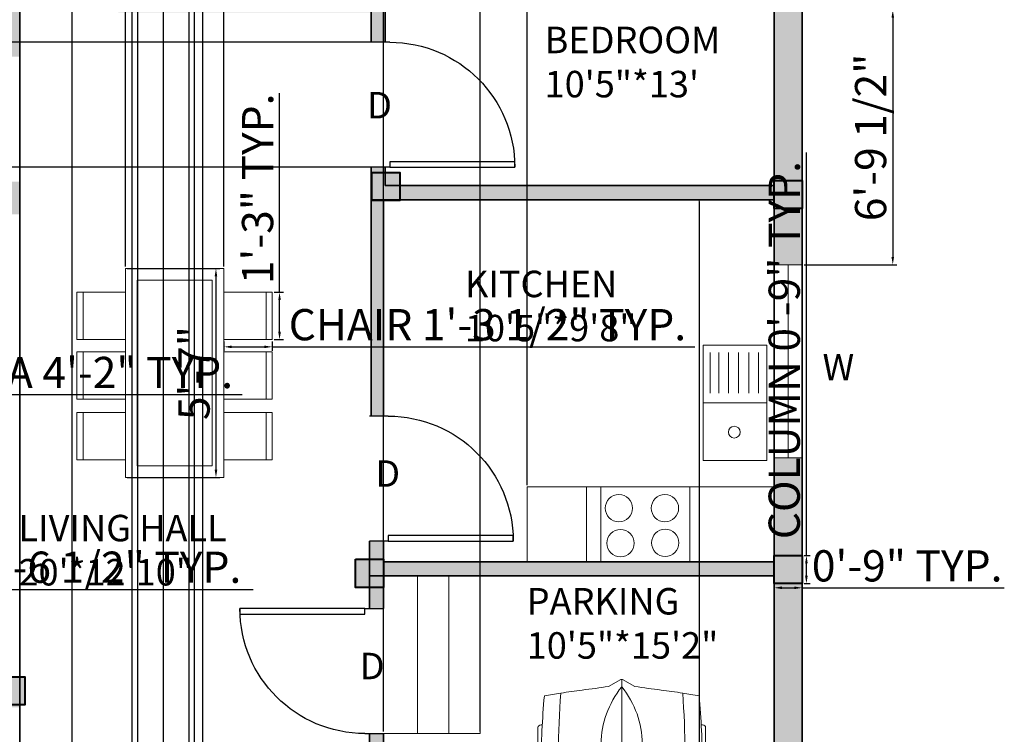
# Model space of a CAD drawing. Units: inches. Extents: x 1801 to 2333, y 2020 to 2714.
# Tile 3 of 4: x 1999 to 2314, y 2274 to 2502. Entities that reach past the tile are written whole.
import ezdxf

# ---------------------------------------------------------------- set-up
doc = ezdxf.new("R2010")
doc.units = ezdxf.units.IN
for name, color, linetype, lineweight in [('A-ANNO-DIMS', 2, 'Continuous', 18), ('A-ANNO-TEXT', 200, 'Continuous', 18), ('A-AREA-IDEN', 200, 'Continuous', 25), ('A-COLS', 7, 'Continuous', 40), ('A-COLS-PATT', 250, 'Continuous', 13), ('A-DOOR', 4, 'Continuous', 25), ('A-EQPM', 8, 'Continuous', 18), ('A-FLOR-CASE', 32, 'Continuous', 18), ('A-FLOR-FIXT', 9, 'Continuous', 18), ('A-FLOR-STRS', 7, 'Continuous', 18), ('A-FURN', 8, 'Continuous', 18), ('A-SITE-VEHI', 8, 'Continuous', 13), ('A-WALL-PATT', 252, 'Continuous', 13), ('WALL', 150, 'Continuous', 35), ('WINDOW', 130, 'Continuous', 18)]:
    doc.layers.add(name, color=color, linetype=linetype, lineweight=lineweight)
doc.styles.get("Standard").update_dxf_attribs({"font": 'arial.ttf'})
doc.dimstyles.new('ISO-25', dxfattribs={"dimtxt": 10, "dimasz": 2.5, "dimexe": 1.25, "dimexo": 0.625, "dimtad": 1, "dimdec": 0, "dimlunit": 4, "dimtxsty": 'Standard', "dimcen": 2.5, "dimadec": 0, "dimazin": 0, "dimtfac": 1, "dimtdec": 0, "dimtmove": 0, "dimatfit": 3, "dimfxl": 1, "dimarcsym": 0})

# ---------------------------------------------------------------- blocks, each defined once
blk = doc.blocks.new('*U2')
for p, q in [((0, 0), (0, -6)), ((40, 0), (40, -6))]:
    blk.add_line(p, q)
blk.add_lwpolyline([(0, 0), (0, 40), (1.75, 40), (1.75, 0)], close=True)
blk.add_arc((0, 0), 40, 0, 90)
blk = doc.blocks.new('*U6')
for p, q in [((21.1, 37.41), (21.1, 36.83)), ((46.55, 38.89), (22.35, 38.89)), ((47.8, 37.39), (47.8, 37.41)), ((135.45, 37.07), (135.45, 37.41)), ((136.7, 38.89), (160.9, 38.89)), ((162.15, 37.41), (162.15, 36.77)), ((87.99, 31.87), (74.76, 35.92)), ((134.31, 35.6), (119.29, 31.78)), ((186.47, -33.5), (186.47, 33.5)), ((188.4, -32.76), (188.4, 32.76)), ((70.03, 31.54), (86.41, 29.35)), ((138.42, 29.35), (157.25, 29.35)), ((186.47, 29.35), (167.01, 29.35)), ((164.52, 26.39), (164.52, -26.39)), ((32.27, 11.63), (36.13, 17.17)), ((36.13, 17.17), (50.94, 17.17)), ((29.77, 9.51), (51.68, 9.51)), ((32.12, 9.51), (32.12, 11.15)), ((58.92, -10.77), (58.92, 10.77)), ((66.55, -10.53), (66.55, 10.53)), ((186.47, -10.53), (186.47, 10.53)), ((3.27, 6.13), (0.1, 0.41)), ((82.74, 8.5), (82.74, -8.5)), ((0, 0), (51.68, 0)), ((0.1, -0.41), (3.27, -6.13)), ((29.77, -9.51), (51.68, -9.51)), ((32.12, -9.51), (32.12, -11.15)), ((32.27, -11.63), (36.13, -17.17)), ((36.13, -17.17), (50.94, -17.17)), ((86.41, -29.35), (70.03, -31.54)), ((87.99, -31.87), (74.76, -35.92)), ((134.31, -35.6), (119.29, -31.78)), ((157.25, -29.35), (138.42, -29.35)), ((167.01, -29.35), (186.47, -29.35)), ((21.1, -37.41), (21.1, -36.83)), ((46.55, -38.89), (22.35, -38.89)), ((47.8, -37.39), (47.8, -37.41)), ((135.45, -37.07), (135.45, -37.41)), ((136.7, -38.89), (160.9, -38.89)), ((162.15, -37.41), (162.15, -36.77))]:
    blk.add_line(p, q)
for centre, major_axis, ratio, start_param, end_param in [((41.19, -490.86), (0, 528.23), 0.842304, 0.00281, 0.075598), ((22.35, 37.41), (0, -1.48), 0.842304, 3.141593, 4.712389), ((64.48, -10555.62), (0, 10593.03), 0.842304, -0.013397, 0.002797), ((46.55, 37.41), (0, 1.48), 0.842304, -1.570796, 0), ((136.7, 37.41), (0, -1.48), 0.842304, 3.141593, 4.712389), ((160.9, 37.41), (0, 1.48), 0.842304, -1.570796, 0), ((180.63, 35.84), (0, 2.22), 0.842304, -0.013017, 1.249894), ((64.48, -10556.36), (0, 10595.31), 0.842304, -0.013397, -0.013017), ((183.98, 32.76), (0, -5.25), 0.842304, 1.570796, 3.128196), ((266.03, -27.52), (0, 313.31), 0.842304, 1.367076, 1.39176), ((64.48, -10555.62), (0, -10591.55), 0.842304, 3.133765, 3.140441), ((183.98, 33.5), (0, -2.96), 0.842304, 1.570796, 3.128196), ((259.18, -27.52), (0, -305.3), 0.842304, 4.528606, 4.561838), ((37.47, -593.96), (0, -623.33), 0.842304, 3.096046, 3.200911), ((134.4, 5.39), (0, -89.78), 0.842304, 4.449482, 4.652344), ((135.29, 5.39), (0, 81.77), 0.842304, 1.245306, 1.50788), ((149.6, 2.8), (0, -79.58), 0.842304, 4.372215, 4.640744), ((95.79, -3666.35), (0, -3698.24), 0.842304, 3.134049, 3.144098), ((17.08, 0), (0, 147.02), 0.842304, 4.511394, 4.913384), ((35.91, 0), (0, 147.02), 0.842304, 4.511394, 4.913384), ((167.01, 26.39), (0, 2.96), 0.842304, 0, 1.570796), ((-204.49, 52.4), (0, -250.96), 0.842304, 1.385369, 1.434372), ((13.04, 17.01), (0, 27.42), 0.842304, 4.435146, 4.718221), ((14.2, 17.01), (0, 27.42), 0.842304, 4.435146, 4.718221), ((50.79, 13.34), (6.34, -0.36), 0.603834, -1.395552, 1.581315), ((29.77, -46.66), (0, 56.17), 0.842304, 0, 0.590319), ((32.75, 11.15), (0, 0.74), 0.842304, 0.879714, 1.570796), ((0.62, 0), (0, -0.74), 0.842304, 4.131459, 5.293319), ((29.77, 46.66), (0, 56.17), 0.842304, 2.551274, 3.141593), ((-204.49, -52.4), (0, 250.96), 0.842304, -1.434372, -1.385369), ((149.6, -2.8), (0, -79.58), 0.842304, -1.499151, -1.230623), ((32.75, -11.15), (0, -0.74), 0.842304, 4.712389, 5.403472), ((13.04, -17.01), (0, -27.42), 0.842304, 1.564964, 1.848039), ((14.2, -17.01), (0, -27.42), 0.842304, 1.564964, 1.848039), ((134.4, -5.39), (0, -89.78), 0.842304, -1.510751, -1.307889), ((135.29, -5.39), (0, -81.77), 0.842304, -1.50788, -1.245306), ((259.18, 27.52), (0, 305.3), 0.842304, 1.721348, 1.754579), ((167.01, -26.39), (0, -2.96), 0.842304, 4.712389, 6.283185), ((266.03, 27.52), (0, 313.31), 0.842304, 1.749832, 1.774517), ((37.47, 593.96), (0, -623.33), 0.842304, -0.059319, 0.045547), ((95.79, 3666.35), (0, -3698.24), 0.842304, -0.002505, 0.007544), ((41.19, 490.86), (0, -528.23), 0.842304, -0.075598, -0.00281), ((64.48, 10555.62), (0, 10593.03), 0.842304, 3.138796, 3.15499), ((64.48, 10555.62), (0, -10591.55), 0.842304, 0.001152, 0.007828), ((183.98, -33.5), (0, 2.96), 0.842304, 3.15499, 4.712389), ((183.98, -32.76), (0, -5.25), 0.842304, 0.013397, 1.570796), ((22.35, -37.41), (0, 1.48), 0.842304, 1.570796, 3.141593), ((46.55, -37.41), (0, -1.48), 0.842304, 0, 1.570796), ((136.7, -37.41), (0, -1.48), 0.842304, -1.570796, 0), ((160.9, -37.41), (0, 1.48), 0.842304, 3.141593, 4.712389), ((180.63, -35.84), (0, -2.22), 0.842304, -1.249894, 0.013017), ((64.48, 10556.36), (0, 10595.31), 0.842304, 3.15461, 3.15499)]:
    blk.add_ellipse(centre, major_axis=major_axis, ratio=ratio, start_param=start_param, end_param=end_param)
at = {"extrusion": (0, 0, -1)}
blk.add_ellipse((50.79, -13.34), major_axis=(6.34, 0.36), ratio=0.603834, start_param=-1.395552, end_param=1.581315, dxfattribs=at)
blk = doc.blocks.new('CHAIR-DINING')
blk.add_line((13.54, 15.15), (13.54, 0))
blk.add_lwpolyline([(0, 15.15), (15.49, 15.15), (15.49, 0), (0, 0)], close=True)
blk = doc.blocks.new('WIN-STANDARD')
blk.add_line((0, 4.5), (61.87, 4.5))
blk.add_lwpolyline([(0, 9), (61.87, 9), (61.87, 0), (0, 0)], close=True)
blk = doc.blocks.new('COLUMN-9X9')
blk.add_lwpolyline([(0, 9), (9, 9), (9, 0), (0, 0)], close=True)
blk = doc.blocks.new('*D16')
at = {"layer": 'A-ANNO-DIMS', "color": 0, "lineweight": -2, "transparency": 16777216}
for p, q in [((2251.04, 2330.92), (2251.04, 2459.93)), ((2250.31, 2330.92), (2252.29, 2330.92)), ((2251.04, 2324.42), (2251.04, 2328.42)), ((2250.31, 2321.92), (2252.29, 2321.92))]:
    blk.add_line(p, q, dxfattribs=at)
at = {"layer": 'A-ANNO-DIMS', "color": 0, "transparency": 16777216}
for points in [[(2250.62, 2328.42), (2251.46, 2328.42), (2251.04, 2330.92)], [(2250.62, 2324.42), (2251.46, 2324.42), (2251.04, 2321.92)]]:
    blk.add_solid(points, dxfattribs=at)
at = {"layer": 'Defpoints', "color": 0, "transparency": 16777216}
for p in [(2249.69, 2330.92), (2251.04, 2330.92), (2249.69, 2321.92)]:
    blk.add_point(p, dxfattribs=at)
at = {"layer": 'A-ANNO-DIMS', "color": 0, "transparency": 16777216, "insert": (2245.24, 2396.68), "char_height": 10, "attachment_point": 5, "rotation": 90}
blk.add_mtext('COLUMN 0\'-9" TYP.', dxfattribs=at)
blk = doc.blocks.new('*D17')
at = {"layer": 'A-ANNO-DIMS', "color": 0, "lineweight": -2, "transparency": 16777216}
for p, q in [((2240.69, 2321.3), (2240.69, 2319.32)), ((2243.19, 2320.57), (2247.19, 2320.57)), ((2249.69, 2321.3), (2249.69, 2319.32)), ((2249.69, 2320.57), (2314.39, 2320.57))]:
    blk.add_line(p, q, dxfattribs=at)
at = {"layer": 'A-ANNO-DIMS', "color": 0, "transparency": 16777216}
for points in [[(2243.19, 2320.99), (2243.19, 2320.15), (2240.69, 2320.57)], [(2247.19, 2320.99), (2247.19, 2320.15), (2249.69, 2320.57)]]:
    blk.add_solid(points, dxfattribs=at)
at = {"layer": 'Defpoints', "color": 0, "transparency": 16777216}
for p in [(2240.69, 2321.92), (2249.69, 2321.92), (2249.69, 2320.57)]:
    blk.add_point(p, dxfattribs=at)
at = {"layer": 'A-ANNO-DIMS', "color": 0, "transparency": 16777216, "insert": (2283.29, 2326.3), "char_height": 10, "attachment_point": 5}
blk.add_mtext('0\'-9" TYP.', dxfattribs=at)
blk = doc.blocks.new('*D24')
at = {"layer": 'A-ANNO-DIMS', "color": 0, "lineweight": -2, "transparency": 16777216}
for p, q in [((2064.57, 2399.42), (2064.57, 2396.48)), ((2080.05, 2399.42), (2080.05, 2396.48)), ((2067.07, 2397.73), (2077.55, 2397.73)), ((2080.05, 2397.73), (2215.29, 2397.73))]:
    blk.add_line(p, q, dxfattribs=at)
at = {"layer": 'A-ANNO-DIMS', "color": 0, "transparency": 16777216}
for points in [[(2067.07, 2398.14), (2067.07, 2397.31), (2064.57, 2397.73)], [(2077.55, 2398.14), (2077.55, 2397.31), (2080.05, 2397.73)]]:
    blk.add_solid(points, dxfattribs=at)
at = {"layer": 'Defpoints', "color": 0, "transparency": 16777216}
for p in [(2064.57, 2400.05), (2080.05, 2400.05), (2080.05, 2397.73)]:
    blk.add_point(p, dxfattribs=at)
at = {"layer": 'A-ANNO-DIMS', "color": 0, "transparency": 16777216, "insert": (2148.92, 2403.53), "char_height": 10, "attachment_point": 5}
blk.add_mtext('CHAIR 1\'-3 1/2" TYP.', dxfattribs=at)
blk = doc.blocks.new('*D25')
at = {"layer": 'A-ANNO-DIMS', "color": 0, "lineweight": -2, "transparency": 16777216}
for p, q in [((2082.38, 2415.2), (2082.38, 2478.96)), ((2080.68, 2415.2), (2083.63, 2415.2)), ((2082.38, 2402.55), (2082.38, 2412.7)), ((2080.68, 2400.05), (2083.63, 2400.05))]:
    blk.add_line(p, q, dxfattribs=at)
at = {"layer": 'A-ANNO-DIMS', "color": 0, "transparency": 16777216}
for points in [[(2081.96, 2412.7), (2082.79, 2412.7), (2082.38, 2415.2)], [(2081.96, 2402.55), (2082.79, 2402.55), (2082.38, 2400.05)]]:
    blk.add_solid(points, dxfattribs=at)
at = {"layer": 'Defpoints', "color": 0, "transparency": 16777216}
for p in [(2080.05, 2415.2), (2082.38, 2415.2), (2080.05, 2400.05)]:
    blk.add_point(p, dxfattribs=at)
at = {"layer": 'A-ANNO-DIMS', "color": 0, "transparency": 16777216, "insert": (2076.64, 2448.33), "char_height": 10, "attachment_point": 5, "rotation": 90}
blk.add_mtext('1\'-3" TYP.', dxfattribs=at)
blk = doc.blocks.new('*D26')
at = {"layer": 'A-ANNO-DIMS', "color": 0, "lineweight": -2, "transparency": 16777216}
for p, q in [((1913.81, 2389.31), (1913.81, 2381.17)), ((1963.87, 2389.31), (1963.87, 2381.17)), ((1916.31, 2382.42), (1961.37, 2382.42)), ((1963.87, 2382.42), (2070.44, 2382.42))]:
    blk.add_line(p, q, dxfattribs=at)
at = {"layer": 'A-ANNO-DIMS', "color": 0, "transparency": 16777216}
for points in [[(1916.31, 2382.84), (1916.31, 2382.01), (1913.81, 2382.42)], [(1961.37, 2382.84), (1961.37, 2382.01), (1963.87, 2382.42)]]:
    blk.add_solid(points, dxfattribs=at)
at = {"layer": 'Defpoints', "color": 0, "transparency": 16777216}
for p in [(1913.81, 2389.93), (1963.87, 2389.93), (1963.87, 2382.42)]:
    blk.add_point(p, dxfattribs=at)
at = {"layer": 'A-ANNO-DIMS', "color": 0, "transparency": 16777216, "insert": (2018.41, 2388.22), "char_height": 10, "attachment_point": 5}
blk.add_mtext('SOFA 4\'-2" TYP.', dxfattribs=at)
blk = doc.blocks.new('*D28')
at = {"layer": 'A-ANNO-DIMS', "color": 0, "lineweight": -2, "transparency": 16777216}
for p, q in [((1886.64, 2317.95), (1886.64, 2321.32)), ((1889.14, 2320.07), (1902.46, 2320.07)), ((1904.96, 2317.95), (1904.96, 2321.32)), ((1904.96, 2320.07), (2073.96, 2320.07))]:
    blk.add_line(p, q, dxfattribs=at)
at = {"layer": 'A-ANNO-DIMS', "color": 0, "transparency": 16777216}
for points in [[(1889.14, 2320.49), (1889.14, 2319.65), (1886.64, 2320.07)], [(1902.46, 2320.49), (1902.46, 2319.65), (1904.96, 2320.07)]]:
    blk.add_solid(points, dxfattribs=at)
at = {"layer": 'Defpoints', "color": 0, "transparency": 16777216}
for p in [(1904.96, 2320.07), (1886.64, 2317.32), (1904.96, 2317.32)]:
    blk.add_point(p, dxfattribs=at)
at = {"layer": 'A-ANNO-DIMS', "color": 0, "transparency": 16777216, "insert": (1990.71, 2325.87), "char_height": 10, "attachment_point": 5}
blk.add_mtext('END TABLE 1\'-6 1/2" TYP.', dxfattribs=at)
blk = doc.blocks.new('*D38')
at = {"layer": 'A-ANNO-DIMS', "color": 0, "lineweight": -2, "transparency": 16777216}
for p, q in [((2250.31, 2505.59), (2279.94, 2505.59)), ((2278.69, 2503.09), (2278.69, 2426.51)), ((2250.31, 2424.01), (2279.94, 2424.01))]:
    blk.add_line(p, q, dxfattribs=at)
at = {"layer": 'A-ANNO-DIMS', "color": 0, "transparency": 16777216}
for points in [[(2278.27, 2503.09), (2279.11, 2503.09), (2278.69, 2505.59)], [(2278.27, 2426.51), (2279.11, 2426.51), (2278.69, 2424.01)]]:
    blk.add_solid(points, dxfattribs=at)
at = {"layer": 'Defpoints', "color": 0, "transparency": 16777216}
for p in [(2249.69, 2505.59), (2249.69, 2424.01), (2278.69, 2424.01)]:
    blk.add_point(p, dxfattribs=at)
at = {"layer": 'A-ANNO-DIMS', "color": 0, "transparency": 16777216, "insert": (2272.89, 2464.8), "char_height": 10, "attachment_point": 5, "rotation": 90}
blk.add_mtext('6\'-9 1/2"', dxfattribs=at)
blk = doc.blocks.new('*D44')
at = {"layer": 'A-ANNO-DIMS', "color": 0, "lineweight": -2, "transparency": 16777216}
for p, q in [((1999.19, 2239.97), (1999.19, 2694.33)), ((2001.69, 2693.08), (2032.69, 2693.08)), ((2035.19, 2239.97), (2035.19, 2694.33))]:
    blk.add_line(p, q, dxfattribs=at)
at = {"layer": 'A-ANNO-DIMS', "color": 0, "transparency": 16777216}
for points in [[(2001.69, 2693.5), (2001.69, 2692.66), (1999.19, 2693.08)], [(2032.69, 2693.5), (2032.69, 2692.66), (2035.19, 2693.08)]]:
    blk.add_solid(points, dxfattribs=at)
at = {"layer": 'Defpoints', "color": 0, "transparency": 16777216}
for p in [(2035.19, 2693.08), (1999.19, 2239.35), (2035.19, 2239.35)]:
    blk.add_point(p, dxfattribs=at)
at = {"layer": 'A-ANNO-DIMS', "color": 0, "transparency": 16777216, "insert": (2017.19, 2698.81), "char_height": 10, "attachment_point": 5}
blk.add_mtext('3\'-0"', dxfattribs=at)
blk = doc.blocks.new('*D45')
at = {"layer": 'A-ANNO-DIMS', "color": 0, "lineweight": -2, "transparency": 16777216}
for p, q in [((2045.19, 2143.97), (2045.19, 2694.33)), ((2047.69, 2693.08), (2052.69, 2693.08)), ((2055.19, 2143.97), (2055.19, 2694.33)), ((2055.19, 2693.08), (2093.29, 2693.08))]:
    blk.add_line(p, q, dxfattribs=at)
at = {"layer": 'A-ANNO-DIMS', "color": 0, "transparency": 16777216}
for points in [[(2047.69, 2693.5), (2047.69, 2692.66), (2045.19, 2693.08)], [(2052.69, 2693.5), (2052.69, 2692.66), (2055.19, 2693.08)]]:
    blk.add_solid(points, dxfattribs=at)
at = {"layer": 'Defpoints', "color": 0, "transparency": 16777216}
for p in [(2055.19, 2693.08), (2045.19, 2143.35), (2055.19, 2143.35)]:
    blk.add_point(p, dxfattribs=at)
at = {"layer": 'A-ANNO-DIMS', "color": 0, "transparency": 16777216, "insert": (2075.49, 2698.81), "char_height": 10, "attachment_point": 5}
blk.add_mtext('0\'-10"', dxfattribs=at)
blk = doc.blocks.new('*D46')
at = {"layer": 'A-ANNO-DIMS', "color": 0, "lineweight": -2, "transparency": 16777216}
for p, q in [((2216.69, 2444.22), (2216.69, 2104.1)), ((2240.69, 2444.22), (2240.69, 2104.1)), ((2219.19, 2105.35), (2238.19, 2105.35)), ((2240.69, 2105.35), (2271.19, 2105.35))]:
    blk.add_line(p, q, dxfattribs=at)
at = {"layer": 'A-ANNO-DIMS', "color": 0, "transparency": 16777216}
for points in [[(2219.19, 2105.76), (2219.19, 2104.93), (2216.69, 2105.35)], [(2238.19, 2105.76), (2238.19, 2104.93), (2240.69, 2105.35)]]:
    blk.add_solid(points, dxfattribs=at)
at = {"layer": 'Defpoints', "color": 0, "transparency": 16777216}
for p in [(2216.69, 2444.85), (2240.69, 2444.85), (2240.69, 2105.35)]:
    blk.add_point(p, dxfattribs=at)
at = {"layer": 'A-ANNO-DIMS', "color": 0, "transparency": 16777216, "insert": (2257.19, 2111.08), "char_height": 10, "attachment_point": 5}
blk.add_mtext('2\'-0"', dxfattribs=at)
blk = doc.blocks.new('*D47')
at = {"layer": 'A-ANNO-DIMS', "color": 0, "lineweight": -2, "transparency": 16777216}
for p, q in [((2053.36, 2604.46), (2053.36, 2104.1)), ((2057.69, 2604.72), (2057.69, 2104.1)), ((2050.86, 2105.35), (2048.36, 2105.35)), ((2053.36, 2105.35), (2057.69, 2105.35)), ((2060.19, 2105.35), (2113.82, 2105.35))]:
    blk.add_line(p, q, dxfattribs=at)
at = {"layer": 'A-ANNO-DIMS', "color": 0, "transparency": 16777216}
for points in [[(2050.86, 2105.76), (2050.86, 2104.93), (2053.36, 2105.35)], [(2060.19, 2105.76), (2060.19, 2104.93), (2057.69, 2105.35)]]:
    blk.add_solid(points, dxfattribs=at)
at = {"layer": 'Defpoints', "color": 0, "transparency": 16777216}
for p in [(2053.36, 2605.08), (2057.69, 2605.35), (2057.69, 2105.35)]:
    blk.add_point(p, dxfattribs=at)
at = {"layer": 'A-ANNO-DIMS', "color": 0, "transparency": 16777216, "insert": (2088.26, 2111.14), "char_height": 10, "attachment_point": 5}
blk.add_mtext('0\'-4 1/2"', dxfattribs=at)
blk = doc.blocks.new('*D48')
at = {"layer": 'A-ANNO-DIMS', "color": 0, "lineweight": -2, "transparency": 16777216}
for p, q in [((2115.56, 2495.25), (1835.44, 2495.25)), ((1836.69, 2457.75), (1836.69, 2492.75)), ((2115.56, 2455.25), (1835.44, 2455.25))]:
    blk.add_line(p, q, dxfattribs=at)
at = {"layer": 'A-ANNO-DIMS', "color": 0, "transparency": 16777216}
for points in [[(1836.27, 2492.75), (1837.11, 2492.75), (1836.69, 2495.25)], [(1836.27, 2457.75), (1837.11, 2457.75), (1836.69, 2455.25)]]:
    blk.add_solid(points, dxfattribs=at)
at = {"layer": 'Defpoints', "color": 0, "transparency": 16777216}
for p in [(1836.69, 2495.25), (2116.19, 2495.25), (2116.19, 2455.25)]:
    blk.add_point(p, dxfattribs=at)
at = {"layer": 'A-ANNO-DIMS', "color": 0, "transparency": 16777216, "insert": (1830.95, 2475.25), "char_height": 10, "attachment_point": 5, "rotation": 90}
blk.add_mtext('3\'-4"', dxfattribs=at)
blk = doc.blocks.new('*D51')
at = {"layer": 'A-ANNO-DIMS', "color": 0, "lineweight": -2, "transparency": 16777216}
for p, q in [((2033.02, 2423.43), (2033.02, 2694.33)), ((2035.52, 2693.08), (2062.07, 2693.08)), ((2064.57, 2423.43), (2064.57, 2694.33)), ((2064.57, 2693.08), (2118.37, 2693.08))]:
    blk.add_line(p, q, dxfattribs=at)
at = {"layer": 'A-ANNO-DIMS', "color": 0, "transparency": 16777216}
for points in [[(2035.52, 2693.5), (2035.52, 2692.66), (2033.02, 2693.08)], [(2062.07, 2693.5), (2062.07, 2692.66), (2064.57, 2693.08)]]:
    blk.add_solid(points, dxfattribs=at)
at = {"layer": 'Defpoints', "color": 0, "transparency": 16777216}
for p in [(2064.57, 2693.08), (2033.02, 2422.8), (2064.57, 2422.8)]:
    blk.add_point(p, dxfattribs=at)
at = {"layer": 'A-ANNO-DIMS', "color": 0, "transparency": 16777216, "insert": (2092.72, 2698.88), "char_height": 10, "attachment_point": 5}
blk.add_mtext('2\'-7 1/2"', dxfattribs=at)
blk = doc.blocks.new('*D52')
at = {"layer": 'A-ANNO-DIMS', "color": 0, "lineweight": -2, "transparency": 16777216}
for p, q in [((2033.64, 2422.8), (2063.27, 2422.8)), ((2062.02, 2420.3), (2062.02, 2358.38)), ((2033.64, 2355.88), (2063.27, 2355.88))]:
    blk.add_line(p, q, dxfattribs=at)
at = {"layer": 'A-ANNO-DIMS', "color": 0, "transparency": 16777216}
for points in [[(2061.6, 2420.3), (2062.43, 2420.3), (2062.02, 2422.8)], [(2061.6, 2358.38), (2062.43, 2358.38), (2062.02, 2355.88)]]:
    blk.add_solid(points, dxfattribs=at)
at = {"layer": 'Defpoints', "color": 0, "transparency": 16777216}
for p in [(2033.02, 2422.8), (2033.02, 2355.88), (2062.02, 2355.88)]:
    blk.add_point(p, dxfattribs=at)
at = {"layer": 'A-ANNO-DIMS', "color": 0, "transparency": 16777216, "insert": (2056.31, 2389.34), "char_height": 10, "attachment_point": 5, "rotation": 90}
blk.add_mtext('5\'-7"', dxfattribs=at)
blk = doc.blocks.new('*D53')
at = {"layer": 'A-ANNO-DIMS', "color": 0, "lineweight": -2, "transparency": 16777216}
for p, q in [((2115.69, 2274.54), (2115.69, 2694.33)), ((2118.19, 2693.08), (2144.09, 2693.08)), ((2146.59, 2274.54), (2146.59, 2694.33))]:
    blk.add_line(p, q, dxfattribs=at)
at = {"layer": 'A-ANNO-DIMS', "color": 0, "transparency": 16777216}
for points in [[(2118.19, 2693.5), (2118.19, 2692.66), (2115.69, 2693.08)], [(2144.09, 2693.5), (2144.09, 2692.66), (2146.59, 2693.08)]]:
    blk.add_solid(points, dxfattribs=at)
at = {"layer": 'Defpoints', "color": 0, "transparency": 16777216}
for p in [(2146.59, 2693.08), (2115.69, 2273.91), (2146.59, 2273.91)]:
    blk.add_point(p, dxfattribs=at)
at = {"layer": 'A-ANNO-DIMS', "color": 0, "transparency": 16777216, "insert": (2131.14, 2698.73), "char_height": 10, "attachment_point": 5}
blk.add_mtext('2\'-7"', dxfattribs=at)
blk = doc.blocks.new('*D54')
at = {"layer": 'A-ANNO-DIMS', "color": 0, "lineweight": -2, "transparency": 16777216}
for p, q in [((2161.67, 2353.47), (2161.67, 2694.33)), ((2164.17, 2693.08), (2238.19, 2693.08)), ((2240.69, 2353.47), (2240.69, 2694.33))]:
    blk.add_line(p, q, dxfattribs=at)
at = {"layer": 'A-ANNO-DIMS', "color": 0, "transparency": 16777216}
for points in [[(2164.17, 2693.5), (2164.17, 2692.66), (2161.67, 2693.08)], [(2238.19, 2693.5), (2238.19, 2692.66), (2240.69, 2693.08)]]:
    blk.add_solid(points, dxfattribs=at)
at = {"layer": 'Defpoints', "color": 0, "transparency": 16777216}
for p in [(2240.69, 2693.08), (2161.67, 2352.85), (2240.69, 2352.85)]:
    blk.add_point(p, dxfattribs=at)
at = {"layer": 'A-ANNO-DIMS', "color": 0, "transparency": 16777216, "insert": (2201.18, 2698.81), "char_height": 10, "attachment_point": 5}
blk.add_mtext('6\'-7"', dxfattribs=at)
blk = doc.blocks.new('*D55')
at = {"layer": 'A-ANNO-DIMS', "color": 0, "lineweight": -2, "transparency": 16777216}
for p, q in [((1999.19, 2604.72), (1999.19, 2104.1)), ((2015.86, 2603.46), (2015.86, 2104.1)), ((2001.69, 2105.35), (2013.36, 2105.35)), ((2015.86, 2105.35), (2068.55, 2105.35))]:
    blk.add_line(p, q, dxfattribs=at)
at = {"layer": 'A-ANNO-DIMS', "color": 0, "transparency": 16777216}
for points in [[(2001.69, 2105.76), (2001.69, 2104.93), (1999.19, 2105.35)], [(2013.36, 2105.76), (2013.36, 2104.93), (2015.86, 2105.35)]]:
    blk.add_solid(points, dxfattribs=at)
at = {"layer": 'Defpoints', "color": 0, "transparency": 16777216}
for p in [(1999.19, 2605.35), (2015.86, 2604.08), (2015.86, 2105.35)]:
    blk.add_point(p, dxfattribs=at)
at = {"layer": 'A-ANNO-DIMS', "color": 0, "transparency": 16777216, "insert": (2043.46, 2111.14), "char_height": 10, "attachment_point": 5}
blk.add_mtext('1\'-4 1/2"', dxfattribs=at)
blk = doc.blocks.new('*D56')
at = {"layer": 'A-ANNO-DIMS', "color": 0, "lineweight": -2, "transparency": 16777216}
for p, q in [((2015.86, 2603.46), (2015.86, 2104.1)), ((2036.86, 2603.46), (2036.86, 2104.1)), ((2018.36, 2105.35), (2034.36, 2105.35)), ((2036.86, 2105.35), (2066.25, 2105.35))]:
    blk.add_line(p, q, dxfattribs=at)
at = {"layer": 'A-ANNO-DIMS', "color": 0, "transparency": 16777216}
for points in [[(2018.36, 2105.76), (2018.36, 2104.93), (2015.86, 2105.35)], [(2034.36, 2105.76), (2034.36, 2104.93), (2036.86, 2105.35)]]:
    blk.add_solid(points, dxfattribs=at)
at = {"layer": 'Defpoints', "color": 0, "transparency": 16777216}
for p in [(2015.86, 2604.08), (2036.86, 2604.08), (2036.86, 2105.35)]:
    blk.add_point(p, dxfattribs=at)
at = {"layer": 'A-ANNO-DIMS', "color": 0, "transparency": 16777216, "insert": (2052.81, 2111.08), "char_height": 10, "attachment_point": 5}
blk.add_mtext('1\'-9"', dxfattribs=at)

msp = doc.modelspace()

# ---------------------------------------------------------------- hatches: boundary and pattern name
at = {"layer": 'A-COLS-PATT'}
h = msp.add_hatch(color=256, dxfattribs=at)
h.dxf.hatch_style = 1
h.paths.add_polyline_path([(1874.69, 2614.35), (1865.69, 2614.35), (1865.69, 2605.35), (1874.69, 2605.35)])
h.paths.add_polyline_path([(2002.83, 2614.35), (1993.83, 2614.35), (1993.83, 2605.35), (2002.83, 2605.35)])
h.paths.add_polyline_path([(2117.06, 2614.35), (2108.06, 2614.35), (2108.06, 2605.35), (2117.06, 2605.35)])
h.paths.add_polyline_path([(2249.69, 2614.35), (2240.69, 2614.35), (2240.69, 2605.35), (2249.69, 2605.35)])
h.paths.add_polyline_path([(1874.69, 2452.27), (1865.69, 2452.27), (1865.69, 2443.27), (1874.69, 2443.27)])
h.paths.add_polyline_path([(1999.19, 2449.12), (1990.19, 2449.12), (1990.19, 2444.85), (1999.19, 2444.85)])
h.paths.add_polyline_path([(1999.19, 2444.85), (1990.19, 2444.85), (1990.19, 2440.12), (1999.19, 2440.12)])
h.paths.add_polyline_path([(2120.9, 2449.35), (2116.19, 2449.35), (2116.19, 2453.56), (2111.9, 2453.56), (2111.9, 2444.85), (2120.9, 2444.85)])
h.paths.add_polyline_path([(2120.9, 2453.56), (2116.19, 2453.56), (2116.19, 2449.35), (2120.9, 2449.35)], flags=17)
h.paths.add_polyline_path([(2249.69, 2451.04), (2240.69, 2451.04), (2240.69, 2442.04), (2249.69, 2442.04)])
h.paths.add_polyline_path([(2249.69, 2330.92), (2240.69, 2330.92), (2240.69, 2321.92), (2249.69, 2321.92)])
h.paths.add_polyline_path([(2115.69, 2329.7), (2111.19, 2329.7), (2111.19, 2324.35), (2115.69, 2324.35)])
h.paths.add_polyline_path([(2115.69, 2324.35), (2111.19, 2324.35), (2111.19, 2320.7), (2115.69, 2320.7)])
h.paths.add_polyline_path([(2111.19, 2329.7), (2106.69, 2329.7), (2106.69, 2320.7), (2111.19, 2320.7), (2111.19, 2324.35)])
h.paths.add_polyline_path([(1999.19, 2291.85), (1991.86, 2291.85), (1991.86, 2287.35), (1994.69, 2287.35), (1994.69, 2283.08), (1999.19, 2283.08)], flags=17)
h.paths.add_polyline_path([(2000.86, 2292.08), (1991.86, 2292.08), (1991.86, 2291.85), (1999.19, 2291.85), (1999.19, 2283.08), (2000.86, 2283.08)])
h.paths.add_polyline_path([(1994.69, 2287.35), (1991.86, 2287.35), (1991.86, 2283.08), (1994.69, 2283.08)], flags=16)
h.paths.add_polyline_path([(1874.69, 2143.35), (1865.69, 2143.35), (1865.69, 2134.35), (1874.69, 2134.35)])
h.paths.add_polyline_path([(1999.19, 2143.35), (1990.19, 2143.35), (1990.19, 2134.35), (1999.19, 2134.35)])
h.paths.add_polyline_path([(2118.63, 2143.35), (2109.63, 2143.35), (2109.63, 2134.35), (2118.63, 2134.35)])
h.paths.add_polyline_path([(2249.69, 2143.35), (2240.69, 2143.35), (2240.69, 2134.35), (2249.69, 2134.35)])
h = msp.add_hatch(color=256, dxfattribs=at)
h.dxf.hatch_style = 1
h.paths.add_polyline_path([(2115.69, 2329.7), (2111.19, 2329.7), (2111.19, 2324.35), (2115.69, 2324.35)])
h.paths.add_polyline_path([(2115.69, 2324.35), (2111.19, 2324.35), (2111.19, 2320.7), (2115.69, 2320.7)])
at = {"layer": 'A-WALL-PATT'}
h = msp.add_hatch(color=256, dxfattribs=at)
h.dxf.hatch_style = 1
h.paths.add_polyline_path([(2067.79, 2614.35), (2044.01, 2614.35), (2044.01, 2605.35), (2053.19, 2605.35), (2067.79, 2605.35)])
h.paths.add_polyline_path([(2057.69, 2605.35), (2053.19, 2605.35), (2053.19, 2509.35), (2040.35, 2509.35), (2030.72, 2509.35), (2030.72, 2504.85), (2040.35, 2504.85), (2057.69, 2504.85), (2111.69, 2504.85), (2111.69, 2509.35), (2057.69, 2509.35)])
h.paths.add_polyline_path([(1999.19, 2605.35), (1994.69, 2605.35), (1994.69, 2490.6), (1999.19, 2490.6)])
h.paths.add_polyline_path([(2116.19, 2605.35), (2111.69, 2605.35), (2111.69, 2550.35), (2111.69, 2535.67, -0.006913), (2112.39, 2535.68), (2116.19, 2535.68), (2116.19, 2551.5)])
h.paths.add_polyline_path([(2116.19, 2510.35), (2112.39, 2510.35), (2111.69, 2510.35), (2111.69, 2495.25), (2116.19, 2495.25)])
h.paths.add_polyline_path([(2115.69, 2273.91), (2111.19, 2273.91), (2111.19, 2143.35), (2115.69, 2143.35)], flags=17)
h.paths.add_polyline_path([(2118.63, 2143.35), (2118.63, 2134.35), (2159.47, 2134.35), (2159.47, 2143.35)])
h.paths.add_polyline_path([(2109.63, 2134.35), (2109.63, 2143.35), (2082.87, 2143.35), (2082.87, 2134.35)])
h.paths.add_polyline_path([(1999.19, 2143.35), (1999.19, 2134.35), (2021.01, 2134.35), (2021.01, 2143.35)])
h.paths.add_polyline_path([(1990.19, 2134.35), (1990.19, 2143.35), (1965.15, 2143.35), (1965.15, 2134.35)])
h.paths.add_polyline_path([(1903.28, 2143.35), (1874.69, 2143.35), (1874.69, 2134.35), (1903.28, 2134.35)])
h.paths.add_polyline_path([(1865.69, 2143.35), (1874.69, 2143.35), (1874.69, 2183.28), (1865.69, 2183.28)])
h.paths.add_polyline_path([(1991.86, 2287.35), (1991.86, 2291.85), (1874.69, 2291.85), (1874.69, 2287.35)])
h.paths.add_polyline_path([(1999.19, 2283.08), (1994.69, 2283.08), (1994.69, 2282.32), (1999.19, 2282.32)])
h.paths.add_polyline_path([(1865.69, 2452.27), (1874.69, 2452.27), (1874.69, 2515.15), (1865.69, 2515.15)])
h.paths.add_polyline_path([(1874.69, 2443.27), (1865.69, 2443.27), (1865.69, 2400.61), (1874.69, 2400.61)])
h.paths.add_polyline_path([(2120.9, 2449.35), (2120.9, 2444.85), (2240.69, 2444.85), (2240.69, 2449.35)])
h.paths.add_polyline_path([(2111.9, 2453.56), (2116.19, 2453.56), (2116.19, 2455.25), (2111.69, 2455.25), (2111.69, 2444.85), (2111.9, 2444.85)])
h.paths.add_polyline_path([(1874.69, 2605.35), (1865.69, 2605.35), (1865.69, 2577.02), (1874.69, 2577.02)])
h.paths.add_polyline_path([(1874.69, 2614.35), (1874.69, 2605.35), (1903.59, 2605.35), (1903.59, 2614.35)])
h = msp.add_hatch(color=256, dxfattribs=at)
h.dxf.hatch_style = 1
h.paths.add_polyline_path([(2249.69, 2505.59), (2240.69, 2505.59), (2240.69, 2451.04), (2249.69, 2451.04)])
h.paths.add_polyline_path([(2249.69, 2442.04), (2240.69, 2442.04), (2240.69, 2424.01), (2249.69, 2424.01)])
h.paths.add_polyline_path([(2249.69, 2362.14), (2240.69, 2362.14), (2240.69, 2330.92), (2249.69, 2330.92)])
h.paths.add_polyline_path([(2249.69, 2321.92), (2240.69, 2321.92), (2240.69, 2143.35), (2249.69, 2143.35)])
h.paths.add_polyline_path([(2240.69, 2143.35), (2214.05, 2143.35), (2214.05, 2134.35), (2240.69, 2134.35)])
h.paths.add_polyline_path([(1874.69, 2282.85), (1865.69, 2282.85), (1865.69, 2245.15), (1874.69, 2245.15)])
h.paths.add_polyline_path([(1874.69, 2338.74), (1865.69, 2338.74), (1865.69, 2291.85), (1874.69, 2291.85)])
h.paths.add_polyline_path([(1990.19, 2449.12), (1999.19, 2449.12), (1999.19, 2450.6), (1994.69, 2450.6), (1994.69, 2449.35), (1874.69, 2449.35), (1874.69, 2444.85), (1990.19, 2444.85)])
h.paths.add_polyline_path([(2141.14, 2614.35), (2117.06, 2614.35), (2117.06, 2605.35), (2141.14, 2605.35)])
h.paths.add_polyline_path([(2108.06, 2614.35), (2102.92, 2614.35), (2102.92, 2605.35), (2108.06, 2605.35)])
h.paths.add_polyline_path([(1993.83, 2614.35), (1965.46, 2614.35), (1965.46, 2605.35), (1993.83, 2605.35)])
h.paths.add_polyline_path([(2008.88, 2614.35), (2002.83, 2614.35), (2002.83, 2605.35), (2008.88, 2605.35)])
h.paths.add_polyline_path([(2107.38, 2466.24), (2120.18, 2466.24), (2120.18, 2483.72), (2107.38, 2483.72)], flags=9)
h.paths.add_polyline_path([(2104.14, 2515.21), (2116.94, 2515.21), (2116.94, 2532.69), (2104.14, 2532.69)], flags=9)
h.paths.add_polyline_path([(2007.5, 2499.97), (2020.3, 2499.97), (2020.3, 2517.44), (2007.5, 2517.44)], flags=9)
h.paths.add_polyline_path([(1985.91, 2461.68), (1998.7, 2461.68), (1998.7, 2479.15), (1985.91, 2479.15)], flags=9)
h.paths.add_polyline_path([(2109.98, 2348.28), (2122.78, 2348.28), (2122.78, 2365.76), (2109.98, 2365.76)], flags=9)
h.paths.add_polyline_path([(1977.13, 2255.51), (1989.93, 2255.51), (1989.93, 2272.99), (1977.13, 2272.99)], flags=9)
h.paths.add_polyline_path([(2063.1, 2540.71), (2101.48, 2540.71), (2101.48, 2560.24), (2063.1, 2560.24)], flags=9)
h.paths.add_polyline_path([(1995.81, 2316.5), (2071.83, 2316.5), (2071.83, 2348.15), (1995.81, 2348.15)], flags=9)
h.paths.add_polyline_path([(2138.31, 2394.68), (2194.97, 2394.68), (2194.97, 2426.33), (2138.31, 2426.33)], flags=9)
h.paths.add_polyline_path([(2163.82, 2472.81), (2229.7, 2472.81), (2229.7, 2504.45), (2163.82, 2504.45)], flags=9)
h.paths.add_polyline_path([(2007.01, 2540.94), (2045.38, 2540.94), (2045.38, 2560.47), (2007.01, 2560.47)], flags=9)
h.paths.add_polyline_path([(1882.98, 2452.95), (1948.86, 2452.95), (1948.86, 2484.59), (1882.98, 2484.59)], flags=9)
h = msp.add_hatch(color=256, dxfattribs=at)
h.dxf.hatch_style = 1
h.paths.add_polyline_path([(2115.69, 2444.85), (2111.69, 2444.85), (2111.69, 2375.54), (2115.69, 2375.54)])
h.paths.add_polyline_path([(2115.69, 2324.35), (2111.19, 2324.35), (2111.19, 2313.91), (2115.69, 2313.91)])
h.paths.add_polyline_path([(1999.19, 2242.32), (1994.69, 2242.32), (1994.69, 2143.35), (1999.19, 2143.35), (1999.19, 2179.35)])
h = msp.add_hatch(color=256, dxfattribs=at)
h.dxf.hatch_style = 1
h.paths.add_polyline_path([(2240.69, 2328.85), (2115.69, 2328.85), (2115.69, 2335.54), (2111.19, 2335.54), (2111.19, 2324.35), (2240.69, 2324.35)])

# ---------------------------------------------------------------- linework, layer by layer
at = {"layer": 'A-EQPM'}
msp.add_lwpolyline([(2185.21, 2352.85), (2213.71, 2352.85), (2213.71, 2328.85), (2185.21, 2328.85)], close=True, dxfattribs=at)
for centre in [(2191.02, 2346.08), (2205.76, 2346.08), (2191.54, 2334.86), (2205.85, 2334.95)]:
    msp.add_circle(centre, 4.37, dxfattribs=at)
at = {"layer": 'A-FLOR-CASE'}
for p, q in [((2240.69, 2444.85), (2216.69, 2444.85)), ((2216.69, 2444.85), (2216.69, 2352.85)), ((2161.67, 2328.85), (2161.67, 2352.85)), ((2161.67, 2352.85), (2216.69, 2352.85)), ((2216.69, 2352.85), (2216.69, 2328.85)), ((2216.69, 2352.85), (2240.69, 2352.85))]:
    msp.add_line(p, q, dxfattribs=at)
msp.add_lwpolyline([(2161.67, 2352.85), (2180.65, 2352.85), (2180.65, 2328.85), (2161.67, 2328.85)], close=True, dxfattribs=at)
at = {"layer": 'A-FLOR-FIXT'}
for p, q in [((2220.21, 2382.85), (2220.21, 2395.9)), ((2223.04, 2382.85), (2223.04, 2395.9)), ((2226.05, 2382.85), (2226.05, 2395.9)), ((2229.31, 2382.85), (2229.31, 2395.9)), ((2232.57, 2382.85), (2232.57, 2395.9)), ((2235.67, 2382.85), (2235.67, 2395.9)), ((2238.42, 2379.79), (2218, 2379.79))]:
    msp.add_line(p, q, dxfattribs=at)
msp.add_lwpolyline([(2218, 2361.31), (2238.42, 2361.31), (2238.42, 2398.26), (2218, 2398.26)], close=True, dxfattribs=at)
msp.add_circle((2227.94, 2370.41), 1.89, dxfattribs=at)
at = {"layer": 'A-FLOR-STRS'}
for p, q in [((2126.59, 2273.91), (2126.59, 2324.35)), ((2136.59, 2273.91), (2136.59, 2324.35)), ((2146.59, 2273.91), (2146.59, 2324.35)), ((2115.69, 2273.91), (2126.59, 2273.91)), ((2126.59, 2273.91), (2146.59, 2273.91))]:
    msp.add_line(p, q, dxfattribs=at)
at = {"layer": 'A-FURN'}
for points in [[(2064.57, 2422.8), (2033.02, 2422.8), (2033.02, 2355.88), (2064.57, 2355.88)], [(2060.81, 2419.04), (2036.78, 2419.04), (2036.78, 2359.64), (2060.81, 2359.64)]]:
    msp.add_lwpolyline(points, close=True, dxfattribs=at)
at = {"layer": 'WALL'}
for p, q in [((2240.69, 2605.35), (2240.69, 2449.35)), ((2111.69, 2495.25), (2111.69, 2511.6)), ((2116.19, 2495.25), (2116.19, 2510.35)), ((2111.69, 2444.85), (2111.69, 2455.25)), ((2116.19, 2449.35), (2116.19, 2455.25)), ((2240.69, 2449.35), (2116.19, 2449.35)), ((2240.69, 2444.85), (2111.69, 2444.85)), ((2111.69, 2375.54), (2111.69, 2444.85)), ((2115.69, 2375.54), (2115.69, 2444.85)), ((2240.69, 2444.85), (2240.69, 2328.85)), ((2111.19, 2324.35), (2111.19, 2335.54)), ((2115.69, 2328.85), (2115.69, 2335.54)), ((2240.69, 2328.85), (2115.69, 2328.85)), ((2240.69, 2324.35), (2111.19, 2324.35)), ((2111.19, 2313.91), (2111.19, 2324.35)), ((2115.69, 2313.91), (2115.69, 2324.35)), ((2111.19, 2143.35), (2111.19, 2273.91)), ((2115.69, 2143.35), (2115.69, 2273.91))]:
    msp.add_line(p, q, dxfattribs=at)
for points in [[(2214.05, 2134.35), (2249.69, 2134.35), (2249.69, 2614.35), (1865.69, 2614.35), (1865.69, 2134.35), (2159.47, 2134.35)], [(2214.05, 2143.35), (2240.69, 2143.35), (2240.69, 2605.35), (1874.69, 2605.35), (1874.69, 2143.35), (2159.47, 2143.35)]]:
    msp.add_lwpolyline(points, dxfattribs=at)

# ---------------------------------------------------------------- block references
at = {"layer": 'A-COLS'}
for p in [(2111.9, 2444.56), (2240.69, 2442.04), (2106.69, 2320.7), (2240.69, 2321.92), (1991.86, 2283.08)]:
    msp.add_blockref('COLUMN-9X9', p, dxfattribs=at)
at = {"layer": 'A-DOOR', "xscale": -1}
for p, rotation in [((2117.69, 2455.25), 270), ((2117.19, 2335.54), 270), ((2109.69, 2313.91), 90)]:
    msp.add_blockref('*U2', p, dxfattribs=dict(at, rotation=rotation))
at = {"layer": 'A-FURN', "extrusion": (0, 0, -1), "zscale": -1}
for p in [(-2033.02, 2400.05), (-2033.02, 2380.96), (-2033.02, 2361.6)]:
    msp.add_blockref('CHAIR-DINING', p, dxfattribs=at)
at = {"layer": 'A-FURN'}
for p in [(2064.57, 2400.05), (2064.57, 2380.96), (2064.57, 2361.6)]:
    msp.add_blockref('CHAIR-DINING', p, dxfattribs=at)
at = {"layer": 'A-SITE-VEHI', "xscale": 0.6906338309990653, "yscale": 0.6906338309990653, "zscale": 0.6906338309990653, "rotation": 270}
msp.add_blockref('*U6', (2191.92, 2291.24), dxfattribs=at)
at = {"layer": 'WINDOW', "rotation": 269.9999999999999}
msp.add_blockref('WIN-STANDARD', (2240.69, 2424.01), dxfattribs=at)

# ---------------------------------------------------------------- texts
at = {"layer": 'A-ANNO-TEXT', "char_height": 8.48, "attachment_point": 1}
for s, insert in [('D', (2110.41, 2479.35)), ('W', (2256.19, 2395.49)), ('D', (2113.01, 2361.39)), ('D', (2108.04, 2299.76))]:
    msp.add_mtext_dynamic_manual_height_columns(s, width=170.2706, gutter_width=42.4, heights=[0], dxfattribs=dict(at, insert=insert))
at = {"layer": 'A-AREA-IDEN', "attachment_point": 1}
for s, insert, char_height in [('BEDROOM\\P10\'5"*13\'', (2167.23, 2500.24), 8.481), ('KITCHEN\\P10\'5"*9\'8"', (2141.72, 2422.11), 8.481), ('LIVING HALL\\P20\'*12\'10"', (1998.8, 2343.93), 8.4809), ('PARKING\\P10\'5"*15\'2"', (2161.5, 2320.49), 8.4809)]:
    msp.add_mtext_dynamic_manual_height_columns(s, width=170.2706, gutter_width=42.4, heights=[0], dxfattribs=dict(at, insert=insert, char_height=char_height))

# ---------------------------------------------------------------- dimensions: what is measured, and where the dimension line sits
at = {"layer": 'A-ANNO-DIMS'}
for base, p1, p2, picture, middle in [((2064.5666, 2693.0804), (2033.0178, 2422.8025), (2064.5666, 2422.8025), '*D51', (2092.7189, 2698.8759)), ((2035.19, 2693.08), (1999.19, 2239.35), (2035.19, 2239.35), '*D44', (2017.19, 2698.81)), ((2055.19, 2693.08), (2045.19, 2143.35), (2055.19, 2143.35), '*D45', (2075.49, 2698.81)), ((2146.59, 2693.08), (2115.69, 2273.91), (2146.59, 2273.91), '*D53', (2131.14, 2698.73)), ((2240.69, 2693.08), (2161.67, 2352.85), (2240.69, 2352.85), '*D54', (2201.18, 2698.81)), ((2015.86, 2105.35), (1999.19, 2605.35), (2015.86, 2604.08), '*D55', (2043.46, 2111.14)), ((2036.86, 2105.35), (2015.86, 2604.08), (2036.86, 2604.08), '*D56', (2052.81, 2111.08)), ((2057.69, 2105.35), (2053.36, 2605.08), (2057.69, 2605.35), '*D47', (2088.26, 2111.14)), ((2240.69, 2105.35), (2216.69, 2444.85), (2240.69, 2444.85), '*D46', (2257.19, 2111.08))]:
    dim = msp.add_linear_dim(base=base, p1=p1, p2=p2, dimstyle='ISO-25', override={"dimdec": 1, "dimlfac": 1, "dimrnd": 0, "dimzin": 1, "dimdsep": 46, "dimlunit": 4, "dimfrac": 2}, dxfattribs=at)
    dim.commit()
    dim.dimension.update_dxf_attribs({"geometry": picture, "text_midpoint": middle})
for base, p1, p2, angle, picture, middle in [((2278.69, 2424.01), (2249.69, 2505.59), (2249.69, 2424.01), 90, '*D38', (2272.89, 2464.8)), ((1836.69, 2495.25), (2116.19, 2455.25), (2116.19, 2495.25), 90, '*D48', (1830.95, 2475.25)), ((2062.02, 2355.88), (2033.02, 2422.8), (2033.02, 2355.88), 270, '*D52', (2056.31, 2389.34))]:
    dim = msp.add_linear_dim(base=base, p1=p1, p2=p2, angle=angle, dimstyle='ISO-25', override={"dimdec": 1, "dimlfac": 1, "dimrnd": 0, "dimzin": 1, "dimdsep": 46, "dimlunit": 4, "dimfrac": 2}, dxfattribs=at)
    dim.commit()
    dim.dimension.update_dxf_attribs({"geometry": picture, "text_midpoint": middle})
for base, p1, p2, text, picture, middle in [((2082.3757, 2415.196), (2080.0528, 2400.0495), (2080.0528, 2415.196), '<> TYP.', '*D25', (2076.6415, 2448.3278)), ((2251.04, 2330.92), (2249.69, 2321.92), (2249.69, 2330.92), 'COLUMN <> TYP.', '*D16', (2245.24, 2396.68))]:
    dim = msp.add_linear_dim(base=base, p1=p1, p2=p2, angle=90, text=text, dimstyle='ISO-25', override={"dimdec": 1, "dimlfac": 1, "dimrnd": 0, "dimzin": 1, "dimdsep": 46, "dimlunit": 4, "dimfrac": 2}, dxfattribs=at)
    dim.commit()
    dim.dimension.update_dxf_attribs({"geometry": picture, "text_midpoint": middle})
for base, p1, p2, text, picture, middle in [((2080.05, 2397.73), (2064.57, 2400.05), (2080.05, 2400.05), 'CHAIR <> TYP.', '*D24', (2148.92, 2403.53)), ((1963.87, 2382.42), (1913.81, 2389.93), (1963.87, 2389.93), 'SOFA <> TYP.', '*D26', (2018.41, 2388.22)), ((1904.96, 2320.07), (1886.64, 2317.32), (1904.96, 2317.32), 'END TABLE <> TYP.', '*D28', (1990.71, 2325.87)), ((2249.69, 2320.57), (2240.69, 2321.92), (2249.69, 2321.92), '<> TYP.', '*D17', (2283.29, 2326.3))]:
    dim = msp.add_linear_dim(base=base, p1=p1, p2=p2, text=text, dimstyle='ISO-25', override={"dimdec": 1, "dimlfac": 1, "dimrnd": 0, "dimzin": 1, "dimdsep": 46, "dimlunit": 4, "dimfrac": 2}, dxfattribs=at)
    dim.commit()
    dim.dimension.update_dxf_attribs({"geometry": picture, "text_midpoint": middle})

doc.saveas('drawing.dxf')
